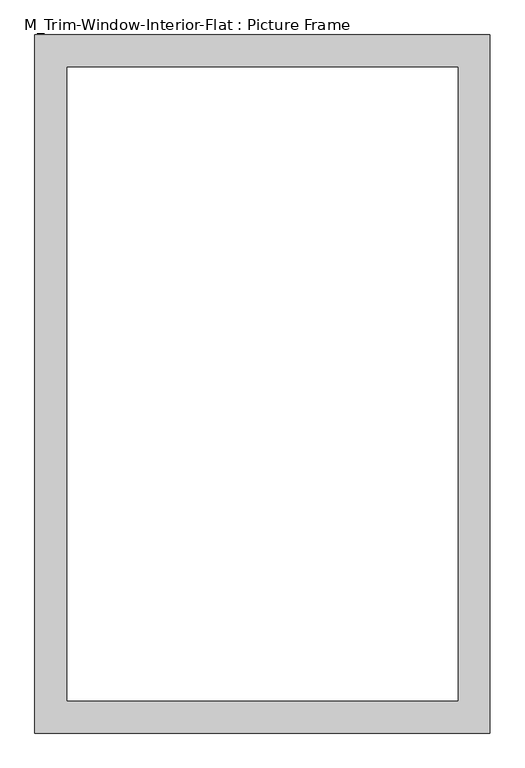
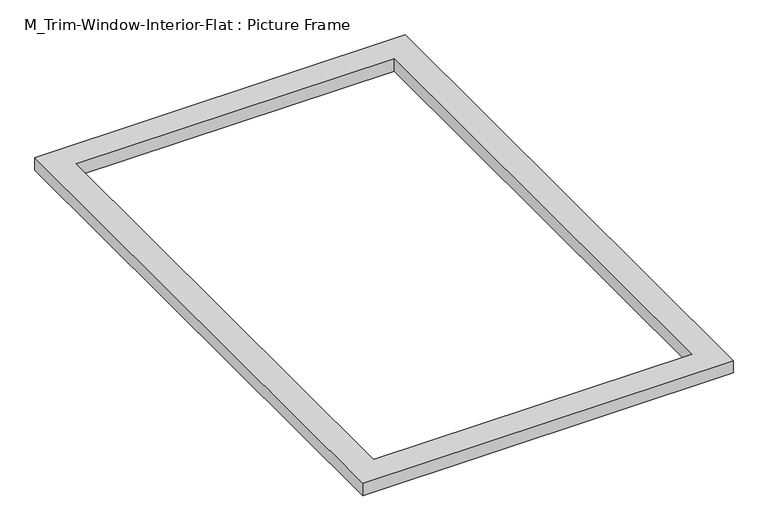
"""IFC4 building model written with IfcOpenShell, lengths in millimetres: proxy geometry, M_Trim-Window-Interior-Flat : Picture Frame."""

from ifc_helpers import new_model, si_unit, origin, origin_with_axes, place, context, project, spatial, polyline, outline, extrude, source, transform, mapped, element, save


def m_trim_window_interior_flat_picture_frame_31bd2320(model_context):
    return source(origin(), model_context, "Body", "SweptSolid", [
        extrude(outline(polyline([(422.3, 47.3), (422.3, -1247.3), (-422.3, -1247.3), (-422.3, 47.3), (422.3, 47.3)]), holes=[polyline([(362.3, -12.7), (-362.3, -12.7), (-362.3, -1187.3), (362.3, -1187.3), (362.3, -12.7)])]), origin_with_axes(), (0.0, 0.0, 1.0), 30.0),
    ])


if __name__ == "__main__":
    model = new_model("IFC4")
    model_context = context("Model", 3, world=origin())
    ifc_project = project(units=[si_unit("LENGTHUNIT", "METRE", prefix="MILLI")], contexts=[model_context])
    site = spatial("IfcSite", under=ifc_project)
    building = spatial("IfcBuilding", under=site)
    placement = place(None, origin())
    m_trim_window_interior_flat_picture_frame_shape = m_trim_window_interior_flat_picture_frame_31bd2320(model_context)
    element("IfcBuildingElementProxy", 1, Name="M_Trim-Window-Interior-Flat : Picture Frame", ObjectType="M_Trim-Window-Interior-Flat : Picture Frame", at=placement, inside=building, context=model_context, shape_type="MappedRepresentation", body=[
        mapped(m_trim_window_interior_flat_picture_frame_shape, transform((0.0, 0.0, 0.0), x_axis=(1.0, 0.0, 0.0), y_axis=(0.0, 1.0, 0.0), z_axis=(0.0, 0.0, 1.0))),
    ])
    save(model, "model.ifc")

# Revit data of these elements
# Type "M_Trim-Window-Interior-Flat : Picture Frame"
#   Trim Thickness_Picture Frame = 0.03 m
#   Trim Width = 0.06 m
#   Trim Thickness_with Sill = 0.02 m
#   Sill Thickness = 0.03 m
#   Opening Width [instance default] = 0.6 m
#   Opening Height [instance default] = 0.9 m
#   Default Elevation = 1.2 m
#   Sill = no
#   Picture Frame = yes
#   Trim Material [instance default] = none
# Element 1 (IfcBuildingElementProxy, "M_Trim-Window-Interior-Flat : Picture Frame")
#   Opening Width = 0.75 m
#   Opening Height = 1.2 m
#   Trim Material = Wood - Stained
#   Materials on its faces: "Wood - Stained"
# Materials
#   "Wood - Stained": class "Wood", colour RGB 224 178 126, transparency 0, Cost = 0
